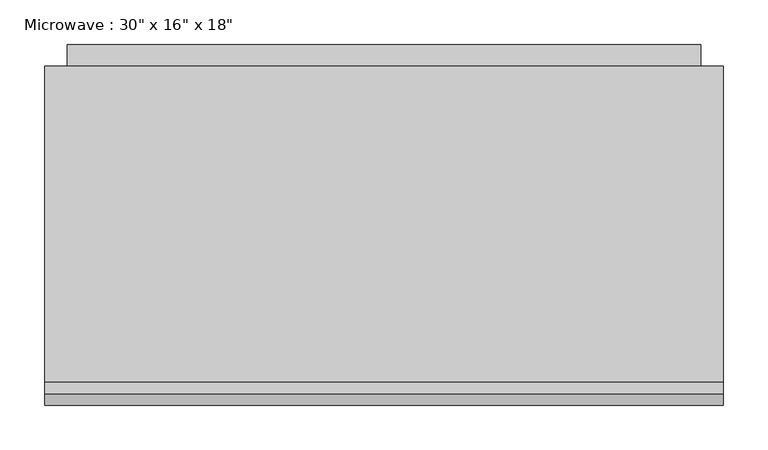
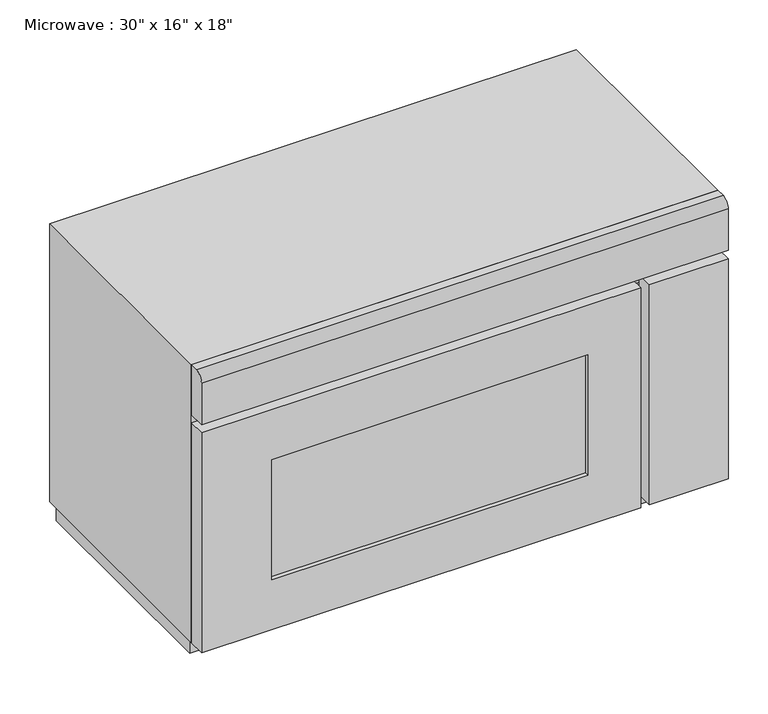
"""IFC4 building model written with IfcOpenShell, lengths in millimetres: proxy geometry."""

from ifc_helpers import new_model, si_unit, point, frame, frame_2d, origin, place, context, project, spatial, polyline, circle_curve, trimmed, segment, composite_curve, outline, extrude, faceted_brep, source, transform, mapped, element, save


def proxy_8a8d5ab2(model_context):
    return source(origin(), model_context, "Body", "SolidModel", [
        extrude(outline(polyline([(678.4897523, -549.9305058), (220.8928773, -549.9305058), (220.8928773, -543.5805058), (678.4897523, -543.5805058), (678.4897523, -549.9305058)])), frame((0.0, 0.0, 1022.35), z_axis=(0.0, 0.0, 1.0), x_axis=(1.0, 0.0, 0.0)), (0.0, 0.0, 1.0), 184.15),
        extrude(outline(polyline([(1282.7, 754.6897523), (1282.7, 119.2928773), (946.15, 119.2928773), (946.15, 754.6897523), (1282.7, 754.6897523)]), holes=[polyline([(1206.5, 678.4897523), (1022.35, 678.4897523), (1022.35, 220.8928773), (1206.5, 220.8928773), (1206.5, 678.4897523)])]), frame((0.0, -556.2805058, 0.0), z_axis=(0.0, 1.0, 0.0), x_axis=(0.0, 0.0, 1.0)), (0.0, 0.0, 1.0), 25.4),
        extrude(outline(polyline([(881.2928773, -556.2805058), (767.3897523, -556.2805058), (767.3897523, -530.8805058), (881.2928773, -530.8805058), (881.2928773, -556.2805058)])), frame((0.0, 0.0, 946.15), z_axis=(0.0, 0.0, 1.0), x_axis=(1.0, 0.0, 0.0)), (0.0, 0.0, 1.0), 336.55),
        extrude(outline(composite_curve([segment(polyline([(-543.5805058, 1371.6), (-530.8805058, 1371.6), (-530.8805058, 1295.4), (-556.2805058, 1295.4), (-556.2805058, 1358.9)]), True, "CONTINUOUS"), segment(trimmed(circle_curve(frame_2d((-543.5805058, 1358.9)), 12.7), [point((-556.2805058, 1358.9))], [point((-543.5805058, 1371.6))], False, "CARTESIAN"), True, "CONTINUOUS")], self_intersect=False)), frame((119.2928773, 0.0, 0.0), z_axis=(1.0, 0.0, 0.0), x_axis=(0.0, 1.0, 0.0)), (0.0, 0.0, 1.0), 762.0),
        extrude(outline(polyline([(-151.0441495, 1346.2), (-151.0441495, 961.946551), (-176.4441495, 936.546551), (-176.4441495, 1346.2), (-151.0441495, 1346.2)])), frame((144.6928773, 0.0, 0.0), z_axis=(1.0, 0.0, 0.0), x_axis=(0.0, 1.0, 0.0)), (0.0, 0.0, 1.0), 711.2),
        faceted_brep([(881.2928773, -175.2805058, 1371.6), (119.2928773, -175.2805058, 1371.6), (119.2928773, -530.8805058, 1371.6), (881.2928773, -530.8805058, 1371.6), (881.2928773, -175.2805058, 946.15), (881.2928773, -530.8805058, 946.15), (119.2928773, -530.8805058, 946.15), (119.2928773, -175.2805058, 946.15), (824.5397523, -530.8805058, 1271.0014904), (824.5397523, -530.8805058, 1020.1764904), (176.0460023, -530.8805058, 1020.1764904), (176.0460023, -530.8805058, 1271.0014904), (824.5397523, -200.6805058, 1271.0014904), (176.0460023, -200.6805058, 1271.0014904), (176.0460023, -200.6805058, 1020.1764904), (824.5397523, -200.6805058, 1020.1764904)], [[[0, 1, 2, 3]], [[4, 5, 6, 7]], [[1, 0, 4, 7]], [[2, 1, 7, 6]], [[3, 2, 6, 5], [8, 9, 10, 11]], [[0, 3, 5, 4]], [[12, 13, 14, 15]], [[12, 15, 9, 8]], [[15, 14, 10, 9]], [[14, 13, 11, 10]], [[13, 12, 8, 11]]]),
        extrude(outline(polyline([(871.7678773, -175.2805058), (871.7678773, -510.2430058), (128.8178773, -510.2430058), (128.8178773, -175.2805058), (871.7678773, -175.2805058)])), frame((0.0, 0.0, 914.4), z_axis=(0.0, 0.0, 1.0), x_axis=(1.0, 0.0, 0.0)), (0.0, 0.0, 1.0), 31.75),
    ])


if __name__ == "__main__":
    model = new_model("IFC4")
    model_context = context("Model", 3, world=origin())
    ifc_project = project(units=[si_unit("LENGTHUNIT", "METRE", prefix="MILLI")], contexts=[model_context])
    site = spatial("IfcSite", under=ifc_project)
    building = spatial("IfcBuilding", under=site)
    placement = place(None, origin())
    proxy_shape = proxy_8a8d5ab2(model_context)
    element("IfcBuildingElementProxy", 1, Name="Microwave : 30\" x 16\" x 18\"", ObjectType="Microwave : 30\" x 16\" x 18\"", at=placement, inside=building, context=model_context, shape_type="MappedRepresentation", body=[
        mapped(proxy_shape, transform((0.0, 0.0, 0.0), x_axis=(1.0, 0.0, 0.0), y_axis=(0.0, 1.0, 0.0), z_axis=(0.0, 0.0, 1.0))),
    ])
    save(model, "model.ifc")

# Revit data of these elements
# Type "Microwave : 30\" x 16\" x 18\""
#   Assembly Code = "E1090400"
#   Depth = 1' - 4"
#   Height = 1' - 6"
#   Width = 2' - 6"
#   Microwave Material = Laminate, Linen, Matte
#   Default Elevation = 0
# Element 1 (IfcBuildingElementProxy, "Microwave : 30\" x 16\" x 18\"")
#   Materials on its faces: "Laminate, Linen, Matte", "Glass"
# Materials
#   "Laminate, Linen, Matte": class "Plastic", colour RGB 249 239 230, transparency 0, Description = "Plastic Laminate - Linen, Matte", Cost = 0
#   "Glass": class "Glass", colour RGB 0 128 192, transparency 0.75, Description = "Soda Lime Glass", Cost = 0
